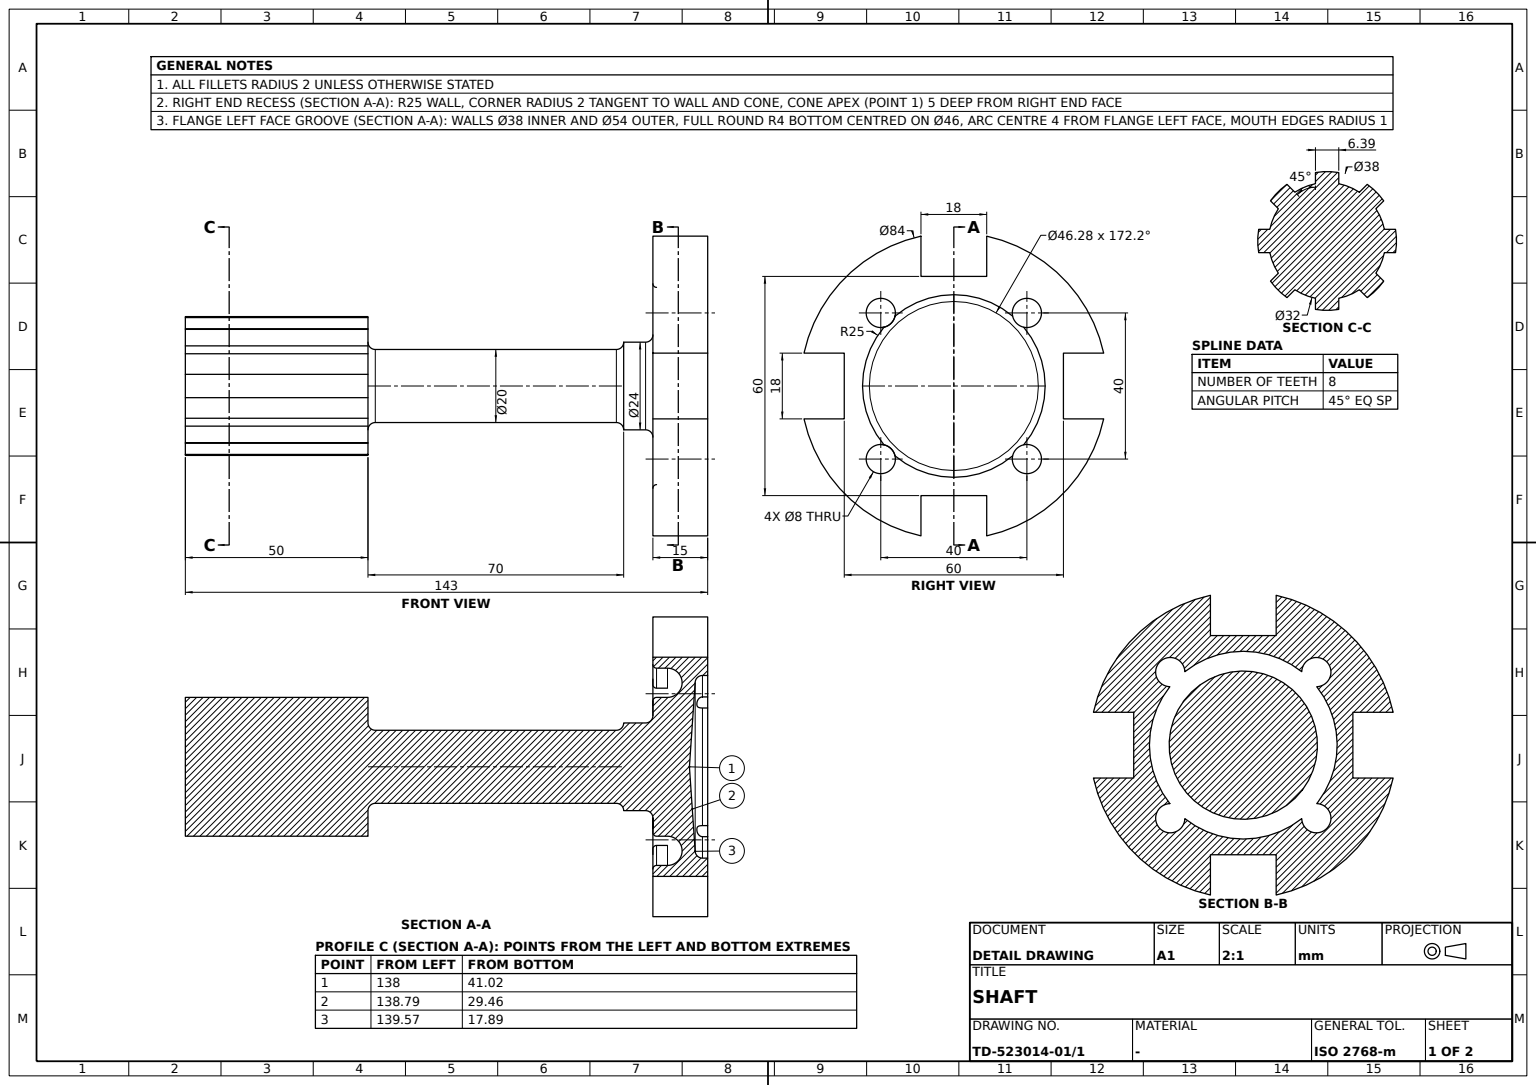
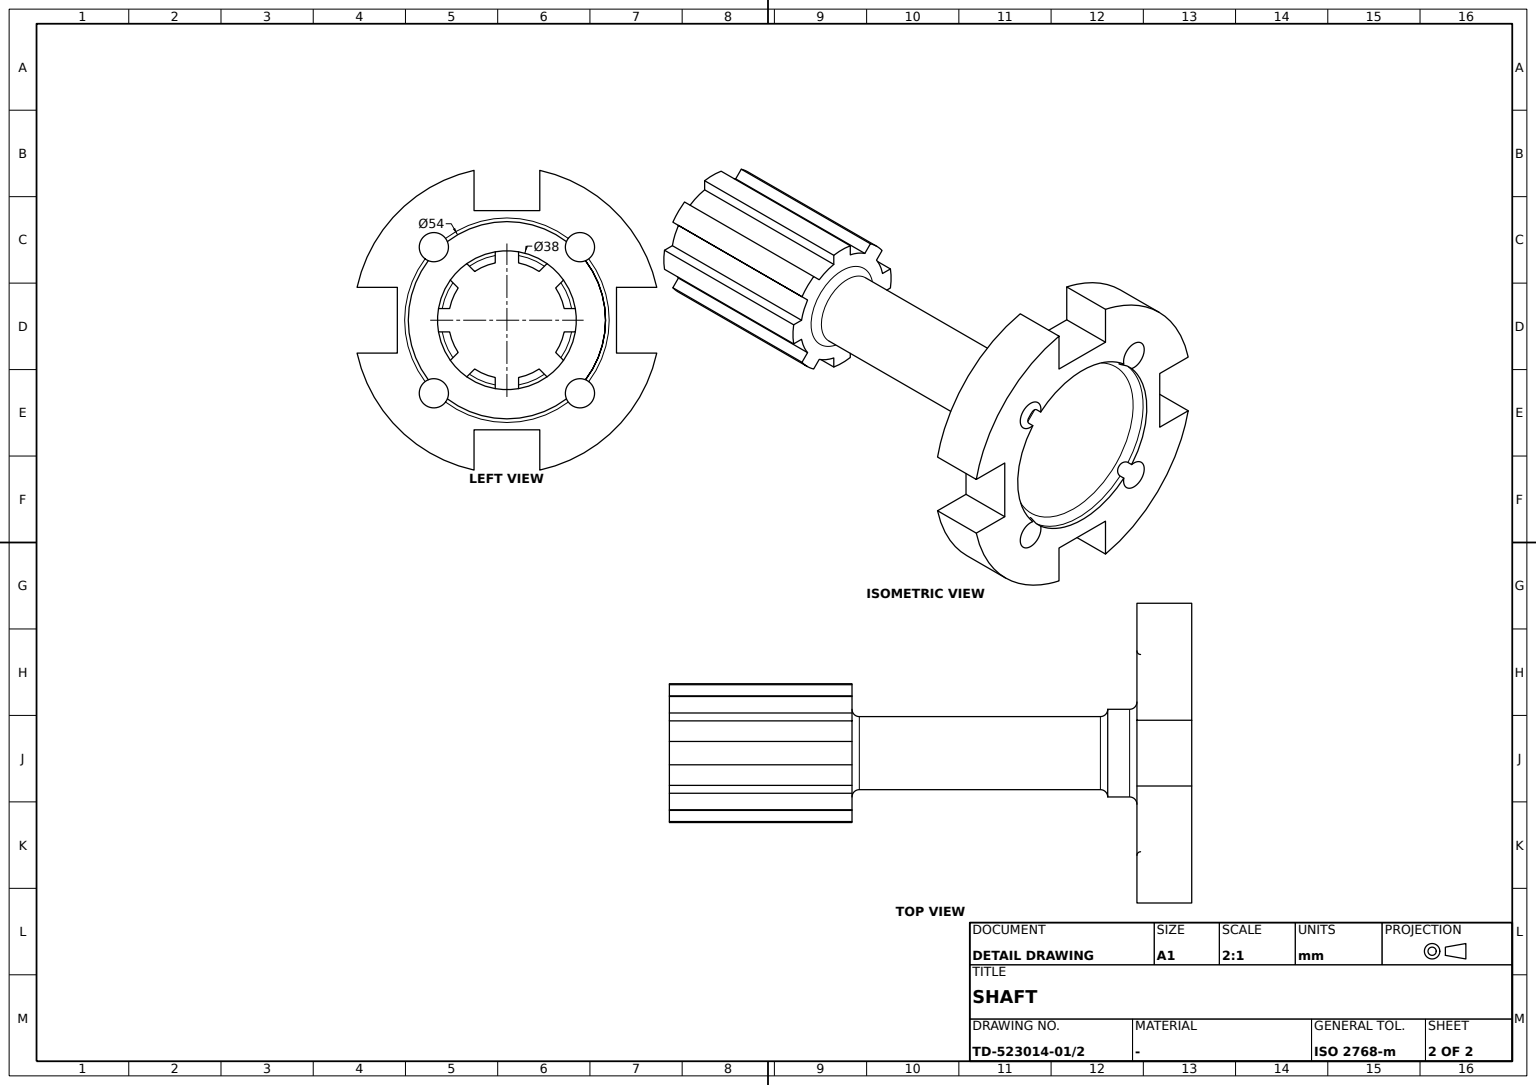
CATIA V5 part; units mm, degrees
sketch "Sketch1" plane through (0, 0, 0) normal (0, 0, 1) x (1, 0, 0)
  line L0 (0, 0) -> (143, 0)
  line L1 (143, 0) -> (143, 42)
  line L2 (143, 42) -> (128, 42)
  line L3 (128, 42) -> (128, 28)
  line L4 (126, 12) -> (120, 12)
  point P0 (120, 12)
  line L5 (120, 12) -> (120, 12)
  point P1 (120, 10)
  line L6 (118, 10) -> (52, 10)
  point P2 (50, 10)
  line L7 (50, 12) -> (50, 16)
  point P3 (50, 16)
  line L8 (50, 16) -> (0, 16)
  point P4 (0, 16)
  line L9 (0, 16) -> (0, 0)
  arc A0 (50, 12) -> (52, 10) centre (52, 12) ccw
  arc A1 (120, 12) -> (118, 10) centre (118, 12) cw
  arc A2 (126, 12) -> (128, 14) centre (126, 14) ccw
  arc A3 (132, 19) -> (132, 27) centre (132, 23) ccw
  point P5 (132, 23)
  line L10 (132, 27) -> (129, 27)
  line L11 (132, 19) -> (129, 19)
  line L12 (128, 18) -> (128, 14)
  point P6 (128, 19)
  arc A4 (128, 28) -> (129, 27) centre (129, 28) ccw
  arc A5 (128, 18) -> (129, 19) centre (129, 18) cw
  dimension "length L0" = 143
  dimension "length L1" = 42
  dimension "length L2" = 15
  dimension "length L8" = 50
  dimension "length L9" = 16
  dimension "distance P2 P3" = 6
  dimension "distance P1 P2" = 70
  dimension "radius A0" = 2
  dimension "distance P0 P1" = 2
  dimension "radius A1" = 2
  dimension "radius A2" = 2
  dimension "radius A3" = 4
  dimension "distance P5 L3" = 4
  dimension "distance P5 L0" = 23
  dimension "radius A4" = 1
  dimension "radius A5" = 1
  constraint horizontal L0 x-axis
  constraint horizontal L2 x-axis
  constraint horizontal L4 x-axis
  constraint horizontal L6 x-axis
  constraint horizontal L8 x-axis
  constraint horizontal L10 x-axis
  constraint vertical L1 y-axis
  constraint vertical L3 y-axis
  constraint vertical L5 y-axis
  constraint vertical L7 y-axis
  constraint vertical L9 y-axis
  constraint vertical L12 y-axis
  constraint coincidence P4 y-axis
  constraint coincidence L7 P2
  constraint coincidence L6 P2
  constraint coincidence L5 P1
  constraint coincidence L6 P1
  constraint coincidence L3 L12
  constraint coincidence L11 P6
  constraint coincidence L12 P6
  constraint tangency A0 L7
  constraint tangency A0 L6
  constraint tangency A1 L5
  constraint tangency A1 L6
  constraint tangency A2 L4
  constraint tangency A2 L3
  constraint tangency L11 A3
  constraint tangency A4 L3
  constraint tangency A4 L10
  constraint tangency A5 L12
  constraint tangency A5 L11
revolve "Shaft1" add sketch "Sketch1" angle 360 about L0
sketch "Sketch2" plane through (0, 0, 0) normal (-1, 0, 0) x (0, -1, 0)
  arc A0 (3.1933, 15.6781) -> (-3.1933, 15.6781) centre (0, 0) ccw
  arc A1 (3.1933, 18.7297) -> (-3.1933, 18.7297) centre (0, 0) ccw
  line L0 (3.1933, 18.7297) -> (3.1933, 15.6781)
  line L1 (-3.1933, 15.6781) -> (-3.1933, 18.7297)
  arc A2 (-8.828, 13.3441) -> (-13.3441, 8.828) centre (0, 0) ccw
  arc A3 (-10.9859, 15.502) -> (-15.502, 10.9859) centre (0, 0) ccw
  line L2 (-10.9859, 15.502) -> (-8.828, 13.3441)
  line L3 (-13.3441, 8.828) -> (-15.502, 10.9859)
  arc A4 (-15.6781, 3.1933) -> (-15.6781, -3.1933) centre (0, 0) ccw
  arc A5 (-18.7297, 3.1933) -> (-18.7297, -3.1933) centre (0, 0) ccw
  line L4 (-18.7297, 3.1933) -> (-15.6781, 3.1933)
  line L5 (-15.6781, -3.1933) -> (-18.7297, -3.1933)
  arc A6 (-13.3441, -8.828) -> (-8.828, -13.3441) centre (0, 0) ccw
  arc A7 (-15.502, -10.9859) -> (-10.9859, -15.502) centre (0, 0) ccw
  line L6 (-15.502, -10.9859) -> (-13.3441, -8.828)
  line L7 (-8.828, -13.3441) -> (-10.9859, -15.502)
  arc A8 (-3.1933, -15.6781) -> (3.1933, -15.6781) centre (0, 0) ccw
  arc A9 (-3.1933, -18.7297) -> (3.1933, -18.7297) centre (0, 0) ccw
  line L8 (-3.1933, -18.7297) -> (-3.1933, -15.6781)
  line L9 (3.1933, -15.6781) -> (3.1933, -18.7297)
  arc A10 (8.828, -13.3441) -> (13.3441, -8.828) centre (0, 0) ccw
  arc A11 (10.9859, -15.502) -> (15.502, -10.9859) centre (0, 0) ccw
  line L10 (10.9859, -15.502) -> (8.828, -13.3441)
  line L11 (13.3441, -8.828) -> (15.502, -10.9859)
  arc A12 (15.6781, -3.1933) -> (15.6781, 3.1933) centre (0, 0) ccw
  arc A13 (18.7297, -3.1933) -> (18.7297, 3.1933) centre (0, 0) ccw
  line L12 (18.7297, -3.1933) -> (15.6781, -3.1933)
  line L13 (15.6781, 3.1933) -> (18.7297, 3.1933)
  arc A14 (13.3441, 8.828) -> (8.828, 13.3441) centre (0, 0) ccw
  arc A15 (15.502, 10.9859) -> (10.9859, 15.502) centre (0, 0) ccw
  line L14 (15.502, 10.9859) -> (13.3441, 8.828)
  line L15 (8.828, 13.3441) -> (10.9859, 15.502)
  dimension "radius A1" = 19
  dimension "radius A0" = 16
  constraint vertical L0 y-axis
  constraint vertical L1 y-axis
  constraint symmetry L1 L0 y-axis
extrude "Pad1" add sketch "Sketch2" against normal blind 50
sketch "Sketch3" plane through (143, 0, 0) normal (1, 0, 0) x (0, 1, 0)
  circle A0 centre (0, 0) radius 42 construction
  arc A1 (9, 41.0244) -> (-9, 41.0244) centre (0, 0) ccw
  line L0 (9, 41.0244) -> (9, 30)
  line L1 (9, 30) -> (-9, 30)
  line L2 (-9, 30) -> (-9, 41.0244)
  point P0 (9, 50)
  point P1 (9, 30)
  point P2 (-9, 41.0244)
  point P3 (9, 41.0244)
  point P4 (-50, 9)
  point P5 (-9, -50)
  point P6 (50, -9)
  line L3 (0, 0) -> (20, 20) construction
  point P7 (20, 20)
  circle A2 centre (20, 20) radius 4
  point P8 (-9, 30)
  circle A3 centre (-20, 20) radius 4
  point P9 (-30, -9)
  circle A4 centre (-20, -20) radius 4
  point P10 (9, -30)
  circle A5 centre (20, -20) radius 4
  point P11 (-30, -9)
  line L4 (-41.0244, 9) -> (-30, 9)
  line L5 (-30, 9) -> (-30, -9)
  line L6 (-30, -9) -> (-41.0244, -9)
  circle A6 centre (0, 0) radius 42 construction
  arc A7 (-41.0244, 9) -> (-41.0244, -9) centre (0, 0) ccw
  point P12 (9, -30)
  line L7 (-9, -41.0244) -> (-9, -30)
  line L8 (-9, -30) -> (9, -30)
  line L9 (9, -30) -> (9, -41.0244)
  arc A8 (-9, -41.0244) -> (9, -41.0244) centre (0, 0) ccw
  circle A9 centre (0, 0) radius 42 construction
  point P13 (30, 9)
  line L10 (41.0244, -9) -> (30, -9)
  line L11 (30, -9) -> (30, 9)
  line L12 (30, 9) -> (41.0244, 9)
  arc A10 (41.0244, -9) -> (41.0244, 9) centre (0, 0) ccw
  circle A11 centre (0, 0) radius 42 construction
  dimension "length L1" = 18
  dimension "distance P0 P1" = 20
  dimension "angle L3 x axis" = 45
  dimension "radius A2" = 4
  dimension "distance origin P7" = 28.2843
  constraint horizontal L1 x-axis
  constraint vertical L0 y-axis
  constraint vertical L2 y-axis
  constraint symmetry L2 L0 y-axis
  constraint coincidence A0 P2
  constraint coincidence A0 P3
extrude "Pocket1" cut sketch "Sketch3" against normal blind 15
sketch "Sketch4" plane through (0, 0, 0) normal (0, 1, 0) x (-1, 0, 0)
  line L0 (-143, 25) -> (-141.5686, 25)
  point P0 (-143, 25)
  point P1 (-139.7, 25)
  line L1 (-143, 25) -> (-143, 0)
  point P2 (-143, 0)
  line L2 (-143, 0) -> (-138, 0)
  line L3 (-138, 0) -> (-139.5732, 23.1357)
  line L4 (-143, -42) -> (-143, 42) construction
  arc A0 (-141.5686, 25) -> (-139.5732, 23.1357) centre (-141.5686, 23) cw
  dimension "length L2" = 5
  dimension "length L1" = 25
  dimension "distance P0 P1" = 3.3
  dimension "radius A0" = 2
  constraint horizontal L0 x-axis
  constraint horizontal L2 x-axis
  constraint coincidence P2 x-axis
  constraint coincidence L1 L4
  constraint coincidence L0 P1
  constraint coincidence L3 P1
  constraint vertical L1 y-axis
  constraint tangency A0 L0
  constraint tangency A0 L3
revolve "Groove1" cut sketch "Sketch4" angle 360 about L2
